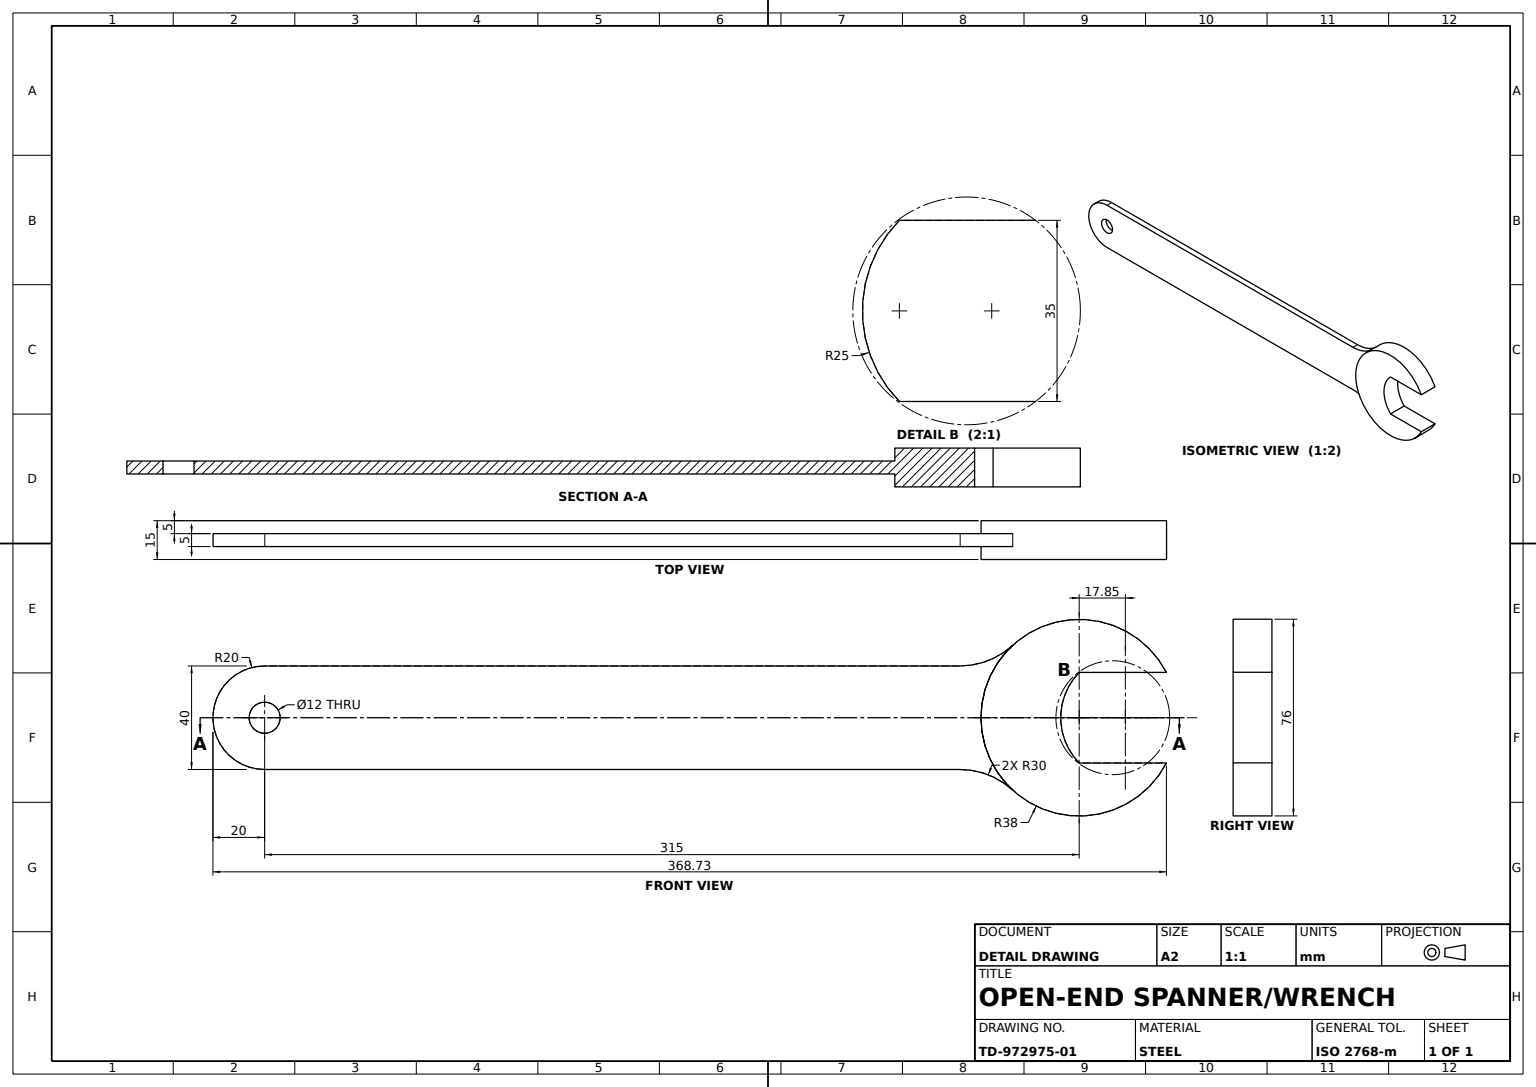
from build123d import *

# Parameters (mm, degrees)
HANDLE_PROFILE_SKETCH_W   = 315
HANDLE_PROFILE_SKETCH_H   = 40
HANDLE_BAR_315X40X5_DEPTH = 5
HANGING_END_SKETCH_R      = 20
ROUNDED_HANGING_END_DEPTH = 5
HEAD_NECK_BOSS_DEPTH      = 5
NECK_TRIM_CUT_R25_DEPTH   = 5
NECK_START                = 5
NECK_FILL_BOSS_A_DEPTH    = 5
NECK_FILL_BOSS_B_DEPTH    = 5
OPEN_START                = -5
OPEN_JAW_HEAD_DEPTH       = 5
HANGING_HOLE_SKETCH_R     = 6
HANGING_HOLE_6_DEPTH      = 15


with BuildPart() as part:
    # Handle Profile Sketch → Handle Bar 315x40x5 (new body)
    with BuildSketch(Plane.XY):
        with Locations((157.5, 20)):
            Rectangle(HANDLE_PROFILE_SKETCH_W, HANDLE_PROFILE_SKETCH_H)
    extrude(amount=HANDLE_BAR_315X40X5_DEPTH)

    # Hanging End Sketch → Rounded Hanging End (add)
    with BuildSketch(Plane.XY.offset(5)):
        with Locations((0, 20)):
            Circle(HANGING_END_SKETCH_R)
    extrude(amount=-ROUNDED_HANGING_END_DEPTH)

    # Neck Profile Sketch → Head Neck Boss (add)
    with BuildSketch(Plane.XY.offset(5)):
        with BuildLine():
            Line((315, 40), (315, 37.5))
            Line((315, 37.5), (348.730549951, 37.5))
            ThreePointArc((348.730549951, 37.5), (316.43745902, 57.972802261), (282.689011157, 40))
            Line((282.689011157, 40), (315, 40))
        make_face()
        with BuildLine():
            Line((348.730549951, 2.5), (315, 2.5))
            Line((315, 2.5), (315, 0))
            Line((315, 0), (282.689011157, 0))
            ThreePointArc((282.689011157, 0), (316.43745902, -17.972802261), (348.730549951, 2.5))
        make_face()
    extrude(amount=-HEAD_NECK_BOSS_DEPTH)

    # Neck Trim Sketch R25 → Neck Trim Cut R25 (cut)
    with BuildSketch(Plane.XY.offset(5)):
        with BuildLine():
            Line((315, 37.5), (315, 2.5))
            ThreePointArc((315, 2.5), (307.853571071, 20), (315, 37.5))
        make_face()
    extrude(amount=-NECK_TRIM_CUT_R25_DEPTH, mode=Mode.SUBTRACT)

    # Neck Fill Sketch A → Neck Fill Boss A (add)
    with BuildSketch(Plane.XY.offset(5).offset(NECK_START)):
        with BuildLine():
            Line((348.730549951, 37.5), (315, 37.5))
            ThreePointArc((315, 37.5), (307.853571071, 20), (315, 2.5))
            Line((315, 2.5), (348.730549951, 2.5))
            ThreePointArc((348.730549951, 2.5), (277, 20), (348.730549951, 37.5))
        make_face()
    extrude(amount=-NECK_FILL_BOSS_A_DEPTH)

    # Neck Fill Sketch B → Neck Fill Boss B (add)
    with BuildSketch(Plane(origin=(0, 0, 0), x_dir=(-1, 0, 0), z_dir=(0, 0, -1))):
        with BuildLine():
            Line((-348.730549951, 37.5), (-315, 37.5))
            ThreePointArc((-315, 37.5), (-307.853571071, 20), (-315, 2.5))
            Line((-315, 2.5), (-348.730549951, 2.5))
            ThreePointArc((-348.730549951, 2.5), (-277, 20), (-348.730549951, 37.5))
        make_face()
    extrude(amount=NECK_FILL_BOSS_B_DEPTH)

    # Jaw Head Sketch → Open Jaw Head (add)
    with BuildSketch(Plane(origin=(0, 0, 0), x_dir=(-1, 0, 0), z_dir=(0, 0, -1)).offset(OPEN_START)):
        with BuildLine():
            Line((-268.913125513, 40), (-282.689011157, 40))
            ThreePointArc((-282.689011157, 40), (-285.697034566, 44.193722673), (-289.245570139, 47.941176471))
            ThreePointArc((-289.245570139, 47.941176471), (-279.827228639, 42.055727726), (-268.913125513, 40))
        make_face()
        with BuildLine():
            Line((-268.913125513, 0), (-282.689011157, 0))
            ThreePointArc((-282.689011157, 0), (-285.697034566, -4.193722673), (-289.245570139, -7.941176471))
            ThreePointArc((-289.245570139, -7.941176471), (-279.827228639, -2.055727726), (-268.913125513, 0))
        make_face()
    extrude(amount=OPEN_JAW_HEAD_DEPTH)

    # Hanging Hole Sketch → Hanging Hole Ø6 (cut)
    with BuildSketch(Plane(origin=(0, 0, 0), x_dir=(-1, 0, 0), z_dir=(0, 0, -1))):
        with Locations((0, 20)):
            Circle(HANGING_HOLE_SKETCH_R)
    extrude(amount=-HANGING_HOLE_6_DEPTH, mode=Mode.SUBTRACT)


solid = part.part
